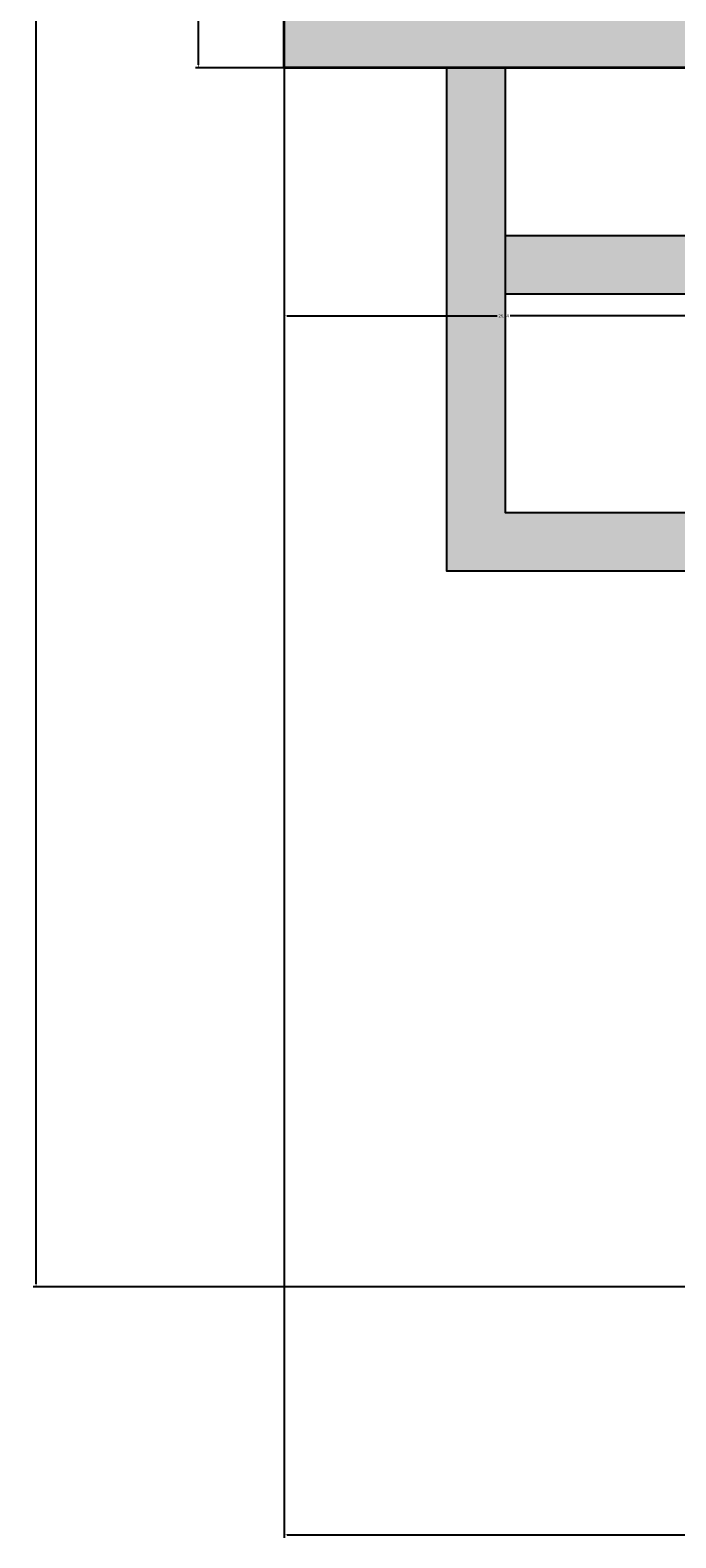
# Model space of a CAD drawing. Units: millimetres. Extents: x -11 to 280, y -4 to 208.
# Tile 1 of 55: x -10 to 28, y -4 to 87. Entities that reach past the tile are written whole.
import ezdxf

# ---------------------------------------------------------------- set-up
doc = ezdxf.new("R2010")
doc.units = ezdxf.units.MM
for name, color, linetype, lineweight in [('M-DIMS', 2, 'Continuous', 18), ('M-HYDR-EQPM', 7, 'Continuous', 35), ('M-HYDR-EQPM-PATT', 252, 'Continuous', 13), ('M-HYDR-RETN', 7, 'Continuous', 25)]:
    doc.layers.add(name, color=color, linetype=linetype, lineweight=lineweight)
doc.layers.add('M-HYDR-RETN-PATT', color=114, linetype='Continuous', lineweight=13, true_color=0x139b48)
doc.styles.get("Standard").update_dxf_attribs({"font": 'arial.ttf'})
doc.dimstyles.get("Standard").update_dxf_attribs({"dimtxt": 0.18, "dimasz": 0.18, "dimexe": 0.18, "dimexo": 0.0625, "dimgap": 0.09, "dimtad": 0, "dimtih": 1, "dimtoh": 1, "dimdec": 4, "dimzin": 0, "dimdsep": 46, "dimtxsty": 'Standard', "dimcen": 0.09, "dimadec": 0, "dimazin": 0, "dimtfac": 1, "dimtdec": 4, "dimtofl": 0, "dimtmove": 0, "dimatfit": 3, "dimfxl": 1, "dimtolj": 1, "dimtzin": 0, "dimarcsym": 0})

# ---------------------------------------------------------------- blocks, each defined once
blk = doc.blocks.new('*D4')
at = {"layer": 'Defpoints', "color": 0, "transparency": 16777216}
for p in [(4.763, 84.426), (266.035, 51.733), (266.035, -3.415)]:
    blk.add_point(p, dxfattribs=at)
at = {"layer": 'M-DIMS', "color": 0, "lineweight": -2, "transparency": 16777216}
for p, q in [((4.763, 84.364), (4.763, -3.595)), ((266.035, 51.67), (266.035, -3.595)), ((4.943, -3.415), (134.934, -3.415)), ((265.855, -3.415), (135.864, -3.415))]:
    blk.add_line(p, q, dxfattribs=at)
at = {"layer": 'M-DIMS', "color": 0, "transparency": 16777216}
for points in [[(4.943, -3.385), (4.943, -3.445), (4.763, -3.415)], [(265.855, -3.385), (265.855, -3.445), (266.035, -3.415)]]:
    blk.add_solid(points, dxfattribs=at)
at = {"layer": 'M-DIMS', "color": 0, "transparency": 16777216, "insert": (135.399, -3.415), "char_height": 0.18, "attachment_point": 5}
blk.add_mtext('\\A1;261.27', dxfattribs=at)
blk = doc.blocks.new('*D5')
at = {"layer": 'Defpoints', "color": 0, "transparency": 16777216}
for p in [(24.759, 192.645), (-10.087, 11.435), (261.686, 11.435)]:
    blk.add_point(p, dxfattribs=at)
at = {"layer": 'M-DIMS', "color": 0, "lineweight": -2, "transparency": 16777216}
for p, q in [((24.696, 192.645), (-10.267, 192.645)), ((-10.087, 192.465), (-10.087, 102.222)), ((-10.087, 11.615), (-10.087, 101.858)), ((261.624, 11.435), (-10.267, 11.435))]:
    blk.add_line(p, q, dxfattribs=at)
at = {"layer": 'M-DIMS', "color": 0, "transparency": 16777216}
for points in [[(-10.117, 192.465), (-10.057, 192.465), (-10.087, 192.645)], [(-10.117, 11.615), (-10.057, 11.615), (-10.087, 11.435)]]:
    blk.add_solid(points, dxfattribs=at)
at = {"layer": 'M-DIMS', "color": 0, "transparency": 16777216, "insert": (-10.087, 102.04), "char_height": 0.18, "attachment_point": 5}
blk.add_mtext('\\A1;181.2', dxfattribs=at)
blk = doc.blocks.new('*D27')
at = {"layer": 'Defpoints', "color": 0, "transparency": 16777216}
for p in [(4.763, 84.426), (31.006, 84.426), (4.763, 69.576)]:
    blk.add_point(p, dxfattribs=at)
at = {"layer": 'M-DIMS', "color": 0, "lineweight": -2, "transparency": 16777216}
for p, q in [((4.763, 84.364), (4.763, 69.396)), ((31.006, 84.364), (31.006, 69.396)), ((4.943, 69.576), (17.49, 69.576)), ((30.826, 69.576), (18.28, 69.576))]:
    blk.add_line(p, q, dxfattribs=at)
at = {"layer": 'M-DIMS', "color": 0, "transparency": 16777216}
for points in [[(4.943, 69.606), (4.943, 69.546), (4.763, 69.576)], [(30.826, 69.606), (30.826, 69.546), (31.006, 69.576)]]:
    blk.add_solid(points, dxfattribs=at)
at = {"layer": 'M-DIMS', "color": 0, "transparency": 16777216, "insert": (17.885, 69.576), "char_height": 0.18, "attachment_point": 5}
blk.add_mtext('\\A1;26.24', dxfattribs=at)
blk = doc.blocks.new('*D28')
at = {"layer": 'Defpoints', "color": 0, "transparency": 16777216}
for p in [(-0.38, 98.021), (14.47, 98.021), (14.47, 84.426)]:
    blk.add_point(p, dxfattribs=at)
at = {"layer": 'M-DIMS', "color": 0, "lineweight": -2, "transparency": 16777216}
for p, q in [((14.408, 98.021), (-0.56, 98.021)), ((-0.38, 97.841), (-0.38, 91.406)), ((-0.38, 84.606), (-0.38, 91.042)), ((14.408, 84.426), (-0.56, 84.426))]:
    blk.add_line(p, q, dxfattribs=at)
at = {"layer": 'M-DIMS', "color": 0, "transparency": 16777216}
for points in [[(-0.41, 97.841), (-0.35, 97.841), (-0.38, 98.021)], [(-0.41, 84.606), (-0.35, 84.606), (-0.38, 84.426)]]:
    blk.add_solid(points, dxfattribs=at)
at = {"layer": 'M-DIMS', "color": 0, "transparency": 16777216, "insert": (-0.38, 91.224), "char_height": 0.18, "attachment_point": 5}
blk.add_mtext('\\A1;13.595', dxfattribs=at)

msp = doc.modelspace()

# ---------------------------------------------------------------- hatches: boundary and pattern name
at = {"layer": 'M-HYDR-EQPM-PATT'}
h = msp.add_hatch(color=256, dxfattribs=at)
h.set_gradient(color1=(69, 84, 165), color2=(0, 0, 255), tint=1)
h.paths.add_polyline_path([(31.0059, 84.4261), (31.0059, 98.0213), (4.7635, 98.0213), (4.7635, 84.4261)])
at = {"layer": 'M-HYDR-RETN-PATT'}
h = msp.add_hatch(color=256, dxfattribs=at)
h.set_gradient(color1=(19, 155, 72), color2=(19, 155, 72), tint=1)
h.paths.add_polyline_path([(17.9701, 159.0814), (29.2015, 159.0814), (29.2015, 162.5814), (14.4701, 162.5814), (14.4701, 98.0213), (17.9701, 98.0213)])
h.paths.add_polyline_path([(17.9701, 84.4261), (14.4701, 84.4261), (14.4701, 54.3099), (156.2446, 54.3099), (156.2446, 57.8099), (17.9701, 57.8099)])
h.paths.add_polyline_path([(120.5137, 74.3991), (17.9701, 74.3991), (17.9701, 70.8991), (120.5137, 70.8991)], flags=17)
h.paths.add_polyline_path([(184.7092, 75.04, 0.4142136), (179.7092, 80.04), (156.2446, 80.04), (156.2446, 57.8099), (156.2446, 54.3099), (156.2446, 43.5991), (159.7446, 43.5991), (159.7446, 57.8099), (159.7446, 76.54), (176.2092, 76.54, -0.4142136), (181.2092, 71.54), (181.2092, 57.8099), (159.7446, 57.8099), (159.7446, 54.3099), (184.7092, 54.3099)])

# ---------------------------------------------------------------- linework, layer by layer
at = {"layer": 'M-HYDR-EQPM'}
msp.add_lwpolyline([(4.7635, 98.0213), (31.0059, 98.0213), (31.0059, 84.4261), (4.7635, 84.4261)], close=True, dxfattribs=at)
at = {"layer": 'M-HYDR-RETN'}
for points in [[(14.4701, 84.4261), (14.4701, 54.3099), (156.2446, 54.3099)], [(17.9701, 84.4261), (17.9701, 57.8099), (156.2446, 57.8099)], [(17.9701, 74.3991), (120.5137, 74.3991)], [(17.9701, 70.8991), (120.5137, 70.8991)]]:
    msp.add_lwpolyline(points, dxfattribs=at)

# ---------------------------------------------------------------- dimensions: what is measured, and where the dimension line sits
at = {"layer": 'M-DIMS'}
for base, p1, p2, angle, override, picture, middle in [((-10.0865, 11.4346), (24.7588, 192.645), (261.6863, 11.4346), 90, {"dimdec": 1, "dimlfac": 1, "dimrnd": 0, "dimzin": 0, "dimdsep": 46, "dimlunit": 2}, '*D5', (-10.0865, 102.0398)), ((-0.3799, 98.0213), (14.4701, 84.4261), (14.4701, 98.0213), 90, {"dimdec": 3, "dimlfac": 1, "dimrnd": 0, "dimzin": 0, "dimdsep": 46, "dimlunit": 2}, '*D28', (-0.3799, 91.2237)), ((4.7635, 69.5761), (31.0059, 84.4261), (4.7635, 84.4261), 180, {"dimdec": 2, "dimlfac": 1, "dimrnd": 0, "dimzin": 0, "dimdsep": 46, "dimlunit": 2}, '*D27', (17.8847, 69.5761))]:
    dim = msp.add_linear_dim(base=base, p1=p1, p2=p2, angle=angle, dimstyle='Standard', override=override, dxfattribs=at)
    dim.commit()
    dim.dimension.update_dxf_attribs({"geometry": picture, "text_midpoint": middle})
dim = msp.add_linear_dim(base=(266.0352, -3.4154), p1=(4.7635, 84.4261), p2=(266.0352, 51.7328), dimstyle='Standard', override={"dimdec": 2, "dimlfac": 1, "dimrnd": 0, "dimzin": 0, "dimdsep": 46, "dimlunit": 2}, dxfattribs=at)
dim.commit()
dim.dimension.update_dxf_attribs({"geometry": '*D4', "text_midpoint": (135.3993, -3.4154)})

doc.saveas('drawing.dxf')
